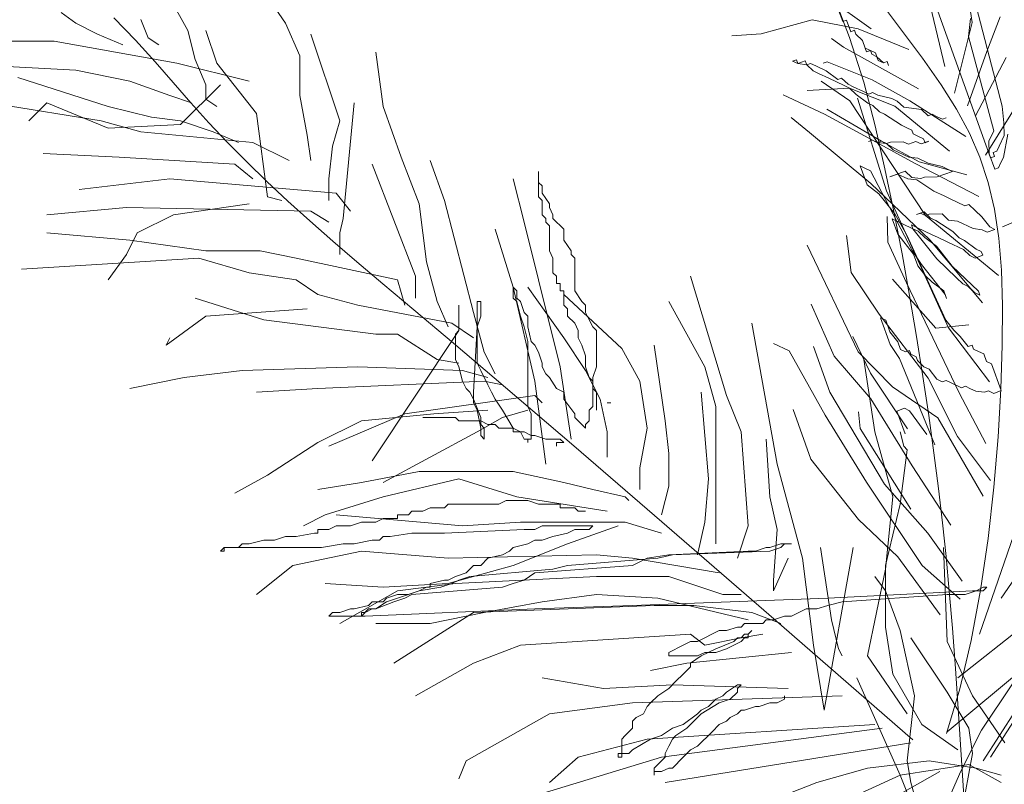
# Model space of a CAD drawing. Units: millimetres. Extents: x 595116 to 630915, y 909473 to 920225.
# Tile 22 of 134: x 629599.598 to 629606.562, y 919171.91 to 919177.315. Entities that reach past the tile are written whole.
import ezdxf

# ---------------------------------------------------------------- set-up
doc = ezdxf.new("R2010")
doc.units = ezdxf.units.MM
doc.layers.add('Dimension', color=3, linetype='Continuous', lineweight=18)
doc.layers.add('L-PLNT', color=85, linetype='Continuous', lineweight=13)
doc.styles.get("Standard").update_dxf_attribs({"font": 'arial.ttf'})
doc.dimstyles.new('ISO-25', dxfattribs={"dimtxt": 9, "dimasz": 6, "dimexe": 1.25, "dimexo": 0.625, "dimtad": 1, "dimlunit": 4, "dimtxsty": 'Standard', "dimcen": 2.5, "dimadec": 0, "dimazin": 0, "dimtfac": 1, "dimtmove": 0, "dimatfit": 3, "dimfxl": 1, "dimarcsym": 0})

# ---------------------------------------------------------------- blocks, each defined once
blk = doc.blocks.new('A$C4FB75ABC')
for p, q in [((2.7169, 3.7399), (2.6018, 4.2172)), ((2.8029, 3.5683), (2.5783, 4.1926)), ((1.2153, 3.9442), (1.2902, 3.808)), ((1.3924, 3.9442), (1.4742, 3.8217)), ((2.7679, 3.8231), (2.7507, 3.9385)), ((2.7636, 3.9026), (2.8247, 3.6653)), ((2.5777, 3.8114), (2.4796, 3.8815)), ((2.5372, 3.7949), (2.5035, 3.8821)), ((2.5794, 3.8826), (2.6314, 3.8136)), ((1.0518, 3.8421), (1.079, 3.8217)), ((2.5166, 3.8462), (2.5244, 3.8247)), ((1.1917, 3.7897), (1.1506, 3.8319)), ((1.2017, 3.8285), (1.2153, 3.7944)), ((2.4664, 3.8281), (2.3706, 3.8017)), ((2.5536, 3.8109), (2.4664, 3.8281)), ((2.5244, 3.8247), (2.5315, 3.8272)), ((2.5315, 3.8272), (2.5393, 3.8057)), ((2.7349, 3.6897), (2.7679, 3.8231)), ((2.7613, 3.7965), (2.7653, 3.8303)), ((2.7957, 3.7683), (2.8207, 3.834)), ((1.079, 3.8217), (1.1199, 3.8012)), ((1.2902, 3.808), (1.3039, 3.7536)), ((1.3243, 3.808), (1.3447, 3.7467)), ((1.4742, 3.8217), (1.5014, 3.7604)), ((2.5393, 3.8057), (2.5464, 3.8083)), ((2.5464, 3.8083), (2.549, 3.8011)), ((2.6486, 3.7721), (2.5536, 3.8109)), ((2.6314, 3.8136), (2.6743, 3.7558)), ((0.9428, 3.7876), (1.0382, 3.7876)), ((1.0382, 3.7876), (1.2698, 3.7467)), ((1.1199, 3.8012), (1.1676, 3.7808)), ((1.2284, 3.7492), (1.1917, 3.7897)), ((1.2153, 3.7944), (1.2357, 3.7808)), ((1.5219, 3.8012), (1.5764, 3.6378)), ((2.3706, 3.8017), (2.3152, 3.798)), ((2.5255, 3.7764), (2.5034, 3.7928)), ((2.5638, 3.7106), (2.5372, 3.7949)), ((2.549, 3.8011), (2.5614, 3.7893)), ((2.5614, 3.7893), (2.5665, 3.775)), ((2.8089, 3.6191), (2.7613, 3.7965)), ((1.6445, 3.7672), (1.6581, 3.665)), ((2.6672, 3.6978), (2.5255, 3.7764)), ((2.5665, 3.775), (2.5763, 3.7704)), ((2.5691, 3.7678), (2.5665, 3.775)), ((2.5763, 3.7704), (2.5691, 3.7678)), ((2.5763, 3.7704), (2.5789, 3.7632)), ((2.586, 3.7658), (2.5763, 3.7704)), ((2.7596, 3.6662), (2.7957, 3.7683)), ((1.2625, 3.7099), (1.2284, 3.7492)), ((1.3039, 3.7536), (1.3243, 3.7059)), ((1.5014, 3.7604), (1.5014, 3.6855)), ((2.4369, 3.7526), (2.4297, 3.7501)), ((2.4297, 3.7501), (2.4394, 3.7455)), ((2.4394, 3.7455), (2.4369, 3.7526)), ((2.4538, 3.7506), (2.4394, 3.7455)), ((2.4564, 3.7435), (2.4538, 3.7506)), ((2.4948, 3.7492), (2.4876, 3.7466)), ((2.58, 3.715), (2.4948, 3.7492)), ((2.5789, 3.7632), (2.5886, 3.7586)), ((2.5886, 3.7586), (2.586, 3.7658)), ((2.5886, 3.7586), (2.5912, 3.7515)), ((2.601, 3.7469), (2.5886, 3.7586)), ((2.5912, 3.7515), (2.601, 3.7469)), ((2.601, 3.7469), (2.6081, 3.7494)), ((2.6081, 3.7494), (2.601, 3.7469)), ((2.6081, 3.7494), (2.6107, 3.7423)), ((2.6107, 3.7423), (2.6081, 3.7494)), ((2.6743, 3.7558), (2.7096, 3.7056)), ((2.7745, 3.6472), (2.8322, 3.7571)), ((0.9496, 3.7399), (1.079, 3.7331)), ((1.079, 3.7331), (1.1812, 3.7127)), ((1.2698, 3.7467), (1.4061, 3.7127)), ((1.3447, 3.7467), (1.4197, 3.6514)), ((2.4394, 3.7455), (2.4564, 3.7435)), ((2.4635, 3.746), (2.4564, 3.7435)), ((2.4564, 3.7435), (2.4687, 3.7317)), ((2.4733, 3.7414), (2.4635, 3.746)), ((2.4687, 3.7317), (2.4785, 3.7271)), ((2.4928, 3.7323), (2.4733, 3.7414)), ((2.5149, 3.7159), (2.4928, 3.7323)), ((0.97, 3.7195), (1.1403, 3.665)), ((1.1812, 3.7127), (1.2562, 3.6855)), ((2.4785, 3.7271), (2.498, 3.7179)), ((2.5376, 3.6754), (2.4836, 3.7127)), ((2.498, 3.7179), (2.5272, 3.7041)), ((2.5221, 3.7185), (2.5149, 3.7159)), ((2.5344, 3.7067), (2.5221, 3.7185)), ((2.6509, 3.6757), (2.58, 3.715)), ((1.2959, 3.6716), (1.2625, 3.7099)), ((1.3515, 3.7059), (1.2766, 3.631)), ((1.3243, 3.7059), (1.3243, 3.6787)), ((2.537, 3.6995), (2.4575, 3.6952)), ((2.5272, 3.7041), (2.537, 3.6995)), ((2.5441, 3.7021), (2.5344, 3.7067)), ((2.537, 3.6995), (2.5493, 3.6877)), ((2.6222, 3.6653), (2.537, 3.6995)), ((2.5637, 3.6929), (2.5441, 3.7021)), ((2.5734, 3.6883), (2.5637, 3.6929)), ((2.5853, 3.6284), (2.5638, 3.7106)), ((2.7096, 3.7056), (2.7388, 3.6597)), ((1.2562, 3.6855), (1.297, 3.6718)), ((1.3243, 3.6787), (1.3447, 3.665)), ((1.5014, 3.6855), (1.5151, 3.6106)), ((2.4899, 3.6502), (2.4119, 3.6869)), ((2.6801, 3.4593), (2.5376, 3.6754)), ((2.5493, 3.6877), (2.5714, 3.6714)), ((2.6067, 3.5058), (2.5519, 3.6806)), ((2.5806, 3.6909), (2.5734, 3.6883)), ((2.5903, 3.6863), (2.5806, 3.6909)), ((2.617, 3.6797), (2.5903, 3.6863)), ((2.6268, 3.6751), (2.617, 3.6797)), ((2.6391, 3.6633), (2.6268, 3.6751)), ((2.7562, 3.6082), (2.6509, 3.6757)), ((2.7932, 3.5729), (2.8652, 3.6879)), ((0.9155, 3.6718), (1.1267, 3.6378)), ((1.0245, 3.6718), (0.9905, 3.6378)), ((1.1403, 3.6242), (1.0245, 3.6718)), ((1.1403, 3.665), (1.2221, 3.6446)), ((1.3299, 3.6341), (1.2959, 3.6716)), ((1.6036, 3.6718), (1.5832, 3.4539)), ((1.6581, 3.665), (1.6922, 3.5697)), ((2.5972, 3.5996), (2.4945, 3.6599)), ((2.5714, 3.6714), (2.5812, 3.6668)), ((2.5812, 3.6668), (2.5935, 3.655)), ((2.5935, 3.655), (2.6032, 3.6504)), ((2.7255, 3.5809), (2.6222, 3.6653)), ((2.673, 3.6593), (2.6391, 3.6633)), ((2.6853, 3.6475), (2.673, 3.6593)), ((2.7388, 3.6597), (2.763, 3.6147)), ((2.8247, 3.6653), (2.8279, 3.634)), ((1.1267, 3.6378), (1.2017, 3.6174)), ((1.2221, 3.6446), (1.2766, 3.6378)), ((1.2766, 3.6378), (1.3379, 3.6174)), ((1.4197, 3.6514), (1.4401, 3.4948)), ((1.5764, 3.6378), (1.5627, 3.5901)), ((2.4618, 3.6157), (2.4274, 3.6439)), ((2.5803, 3.6016), (2.4899, 3.6502)), ((2.6032, 3.6504), (2.6351, 3.6295)), ((2.6925, 3.6501), (2.6853, 3.6475)), ((2.7022, 3.6455), (2.6925, 3.6501)), ((2.712, 3.6409), (2.7022, 3.6455)), ((2.7192, 3.6435), (2.712, 3.6409)), ((1.2766, 3.631), (1.1403, 3.6242)), ((1.365, 3.5971), (1.3299, 3.6341)), ((2.6037, 3.5475), (2.5853, 3.6284)), ((2.6351, 3.6295), (2.6448, 3.6249)), ((2.6448, 3.6249), (2.6546, 3.6203)), ((2.6546, 3.6203), (2.6572, 3.6131)), ((2.7998, 3.5996), (2.8089, 3.6191)), ((2.8279, 3.634), (2.8285, 3.6099)), ((1.2017, 3.6174), (1.4129, 3.5969)), ((1.3379, 3.6174), (1.3856, 3.5969)), ((1.5151, 3.6106), (1.5219, 3.5629)), ((2.5774, 3.5196), (2.4618, 3.6157)), ((2.5803, 3.6016), (2.5731, 3.5991)), ((2.5731, 3.5991), (2.5803, 3.6016)), ((2.5901, 3.597), (2.5803, 3.6016)), ((2.5803, 3.6016), (2.5901, 3.597)), ((2.6609, 3.5577), (2.5803, 3.6016)), ((2.5972, 3.5996), (2.5901, 3.597)), ((2.607, 3.595), (2.5972, 3.5996)), ((2.6681, 3.5603), (2.5972, 3.5996)), ((2.6572, 3.6131), (2.6669, 3.6085)), ((2.6669, 3.6085), (2.6767, 3.6039)), ((2.6864, 3.5993), (2.6721, 3.5942)), ((2.6767, 3.6039), (2.6793, 3.5967)), ((2.6793, 3.5967), (2.6864, 3.5993)), ((2.763, 3.6147), (2.7827, 3.5691)), ((2.8003, 3.5755), (2.7998, 3.5996)), ((2.8285, 3.6099), (2.8193, 3.5904)), ((2.8356, 3.6125), (2.827, 3.5688)), ((1.4014, 3.5604), (1.365, 3.5971)), ((1.4129, 3.5969), (1.481, 3.5629)), ((1.5627, 3.5901), (1.5559, 3.5288)), ((2.5901, 3.597), (2.607, 3.595)), ((2.6142, 3.5976), (2.607, 3.595)), ((2.607, 3.595), (2.6193, 3.5833)), ((2.6383, 3.5982), (2.6142, 3.5976)), ((2.6193, 3.5833), (2.6486, 3.5695)), ((2.648, 3.5936), (2.6383, 3.5982)), ((2.6623, 3.5987), (2.648, 3.5936)), ((2.6721, 3.5942), (2.6623, 3.5987)), ((2.8193, 3.5904), (2.8147, 3.5806)), ((1.0177, 3.5765), (1.1608, 3.5697)), ((1.1608, 3.5697), (1.3788, 3.5561)), ((1.6922, 3.5697), (1.7263, 3.4812)), ((1.7467, 3.5629), (1.7739, 3.488)), ((2.6486, 3.5695), (2.6655, 3.5675)), ((2.6655, 3.5675), (2.685, 3.5583)), ((2.7827, 3.5691), (2.7983, 3.5216)), ((2.8107, 3.5468), (2.8003, 3.5755)), ((2.8101, 3.5709), (2.8029, 3.5683)), ((2.8147, 3.5806), (2.8075, 3.578)), ((2.8075, 3.578), (2.8101, 3.5709)), ((2.827, 3.5688), (2.8224, 3.5591)), ((1.3788, 3.5561), (1.4129, 3.5288)), ((1.4393, 3.5237), (1.4014, 3.5604)), ((1.6377, 3.5561), (1.7194, 3.345)), ((2.5671, 3.5483), (2.5573, 3.5529)), ((2.5573, 3.5529), (2.5703, 3.517)), ((2.5769, 3.5437), (2.5671, 3.5483)), ((2.6552, 3.3935), (2.5769, 3.5437)), ((2.6204, 3.467), (2.6037, 3.5475)), ((2.7805, 3.4954), (2.6609, 3.5577)), ((2.7579, 3.5359), (2.6681, 3.5603)), ((2.685, 3.5583), (2.7117, 3.5517)), ((2.7117, 3.5517), (2.7214, 3.5471)), ((2.7214, 3.5471), (2.7312, 3.5425)), ((2.8178, 3.5493), (2.8107, 3.5468)), ((2.8224, 3.5591), (2.8178, 3.5493)), ((1.0858, 3.5084), (1.2562, 3.5288)), ((1.2562, 3.5288), (1.5696, 3.5016)), ((1.5559, 3.5288), (1.5559, 3.488)), ((1.9034, 3.5288), (1.9238, 3.4471)), ((1.9511, 3.4948), (1.9511, 3.5425)), ((1.9511, 3.5425), (1.9511, 3.522)), ((2.642, 3.5428), (2.6133, 3.5325)), ((2.6133, 3.5325), (2.6276, 3.5376)), ((2.6276, 3.5376), (2.6471, 3.5284)), ((2.6543, 3.531), (2.642, 3.5428)), ((2.6471, 3.5284), (2.6641, 3.5264)), ((2.6712, 3.529), (2.6543, 3.531)), ((2.6641, 3.5264), (2.6959, 3.5055)), ((2.6784, 3.5316), (2.6712, 3.529)), ((2.7025, 3.5321), (2.6784, 3.5316)), ((2.7312, 3.5425), (2.7025, 3.5321)), ((1.4788, 3.4868), (1.4393, 3.5237)), ((1.9511, 3.522), (1.9579, 3.5152)), ((1.9579, 3.5152), (1.9579, 3.5016)), ((2.5703, 3.517), (2.5924, 3.5006)), ((2.6885, 3.4136), (2.5774, 3.5196)), ((2.7983, 3.5216), (2.81, 3.4712)), ((1.4401, 3.4948), (1.4674, 3.488)), ((1.5696, 3.5016), (1.5968, 3.4676)), ((1.7739, 3.488), (1.8285, 3.2769)), ((1.9579, 3.488), (1.9511, 3.4948)), ((1.9579, 3.5016), (1.9715, 3.4812)), ((1.9579, 3.4608), (1.9579, 3.488)), ((2.5924, 3.5006), (2.6222, 3.4627)), ((2.7237, 3.248), (2.6067, 3.5058)), ((2.6959, 3.5055), (2.7154, 3.4963)), ((2.7154, 3.4963), (2.7252, 3.4917)), ((2.7252, 3.4917), (2.7544, 3.4779)), ((2.8253, 3.4385), (2.9518, 3.4922)), ((1.0245, 3.4608), (1.1744, 3.4744)), ((1.1744, 3.4744), (1.5219, 3.4676)), ((1.4061, 3.4812), (1.263, 3.4608)), ((1.5201, 3.4494), (1.4788, 3.4868)), ((1.7263, 3.4812), (1.7399, 3.3722)), ((1.9715, 3.4812), (1.9715, 3.4744)), ((1.9715, 3.4744), (1.9783, 3.4608)), ((2.7544, 3.4779), (2.7616, 3.4805)), ((2.7616, 3.4805), (2.774, 3.4687)), ((2.81, 3.4712), (2.8183, 3.4166)), ((1.263, 3.4608), (1.1949, 3.4267)), ((1.5219, 3.4676), (1.5559, 3.4471)), ((1.5832, 3.4539), (1.5764, 3.4267)), ((1.9647, 3.4539), (1.9579, 3.4608)), ((1.9647, 3.4471), (1.9647, 3.4539)), ((1.9783, 3.4608), (1.9783, 3.4539)), ((1.9783, 3.4539), (1.9988, 3.4335)), ((2.609, 3.4093), (2.6078, 3.4576)), ((2.6566, 3.4346), (2.6176, 3.453)), ((2.6176, 3.453), (2.6279, 3.4243)), ((2.636, 3.3873), (2.6204, 3.467)), ((2.6222, 3.4627), (2.6449, 3.4222)), ((2.6632, 3.4613), (2.6776, 3.4664)), ((2.6704, 3.4639), (2.6632, 3.4613)), ((2.6801, 3.4593), (2.6704, 3.4639)), ((2.6776, 3.4664), (2.6899, 3.4547)), ((2.6873, 3.4618), (2.6801, 3.4593)), ((2.8178, 3.3467), (2.6801, 3.4593)), ((2.7114, 3.4624), (2.6873, 3.4618)), ((2.6899, 3.4547), (2.6996, 3.4501)), ((2.7237, 3.4506), (2.7114, 3.4624)), ((2.774, 3.4687), (2.7863, 3.4569)), ((2.7863, 3.4569), (2.8012, 3.438)), ((1.5633, 3.4112), (1.5201, 3.4494)), ((1.8693, 3.4335), (1.9034, 3.3246)), ((1.9238, 3.4471), (1.9511, 3.3382)), ((1.9715, 3.4403), (1.9647, 3.4471)), ((1.9715, 3.3927), (1.9715, 3.4403)), ((1.9988, 3.4335), (1.9988, 3.4131)), ((2.6638, 3.4372), (2.654, 3.4418)), ((2.654, 3.4418), (2.6566, 3.4346)), ((2.6566, 3.4346), (2.6664, 3.43)), ((2.6865, 3.3967), (2.6566, 3.4346)), ((2.693, 3.4234), (2.6638, 3.4372)), ((2.6996, 3.4501), (2.7315, 3.4291)), ((2.7407, 3.4486), (2.7237, 3.4506)), ((2.7699, 3.4348), (2.7407, 3.4486)), ((2.7869, 3.4328), (2.7699, 3.4348)), ((2.7966, 3.4282), (2.7869, 3.4328)), ((2.811, 3.4334), (2.7966, 3.4282)), ((2.8012, 3.438), (2.811, 3.4334)), ((1.0245, 3.4267), (1.1812, 3.4131)), ((1.1949, 3.4267), (1.1744, 3.3858)), ((1.5764, 3.4267), (1.5764, 3.3858)), ((2.5404, 3.3522), (2.5315, 3.422)), ((2.6279, 3.4243), (2.6578, 3.3864)), ((2.6449, 3.4222), (2.7186, 3.2624)), ((2.6664, 3.43), (2.6787, 3.4182)), ((2.6787, 3.4182), (2.7008, 3.4019)), ((2.7028, 3.4188), (2.693, 3.4234)), ((2.7223, 3.4096), (2.7028, 3.4188)), ((2.7315, 3.4291), (2.7438, 3.4173)), ((2.7438, 3.4173), (2.7536, 3.4127)), ((2.8183, 3.4166), (2.8233, 3.3565)), ((1.1812, 3.4131), (1.3243, 3.3927)), ((1.6088, 3.3721), (1.5633, 3.4112)), ((1.9988, 3.4131), (2.0124, 3.3927)), ((2.5536, 3.203), (2.4572, 3.4034)), ((2.6446, 3.333), (2.609, 3.4093)), ((2.7014, 3.3777), (2.6865, 3.3967)), ((2.7877, 3.2953), (2.6885, 3.4136)), ((2.7008, 3.4019), (2.7306, 3.364)), ((2.7516, 3.3958), (2.7223, 3.4096)), ((2.7639, 3.384), (2.7516, 3.3958)), ((2.7536, 3.4127), (2.7757, 3.3964)), ((2.7757, 3.3964), (2.7854, 3.3918)), ((0.9768, 3.3586), (1.3107, 3.379)), ((1.1744, 3.3858), (1.1403, 3.3382)), ((1.3107, 3.379), (1.4061, 3.3518)), ((1.3243, 3.3927), (1.4265, 3.3927)), ((1.4265, 3.3927), (1.4946, 3.379)), ((1.4946, 3.379), (1.6854, 3.3382)), ((1.9783, 3.379), (1.9715, 3.3927)), ((1.9783, 3.3518), (1.9783, 3.379)), ((2.0124, 3.3927), (2.0124, 3.3858)), ((2.0124, 3.3858), (2.0192, 3.379)), ((2.0192, 3.379), (2.0192, 3.3178)), ((2.6503, 3.3086), (2.636, 3.3873)), ((2.6727, 3.3674), (2.6552, 3.3935)), ((2.6578, 3.3864), (2.6655, 3.3648)), ((2.7384, 3.3424), (2.7014, 3.3777)), ((2.7737, 3.3794), (2.7639, 3.384)), ((2.788, 3.3846), (2.7737, 3.3794)), ((2.7854, 3.3918), (2.788, 3.3846)), ((1.6577, 3.3307), (1.6088, 3.3721)), ((1.7399, 3.3722), (1.7603, 3.2973)), ((2.6655, 3.3648), (2.6804, 3.3459)), ((2.7174, 3.3106), (2.6727, 3.3674)), ((2.7306, 3.364), (2.743, 3.3522)), ((1.4061, 3.3518), (1.4946, 3.3382)), ((1.7194, 3.345), (1.7194, 3.3041)), ((1.9851, 3.345), (1.9783, 3.3518)), ((1.9851, 3.3314), (1.9851, 3.345)), ((2.2372, 3.345), (2.3054, 3.1203)), ((2.5929, 3.2739), (2.5404, 3.3522)), ((2.6997, 3.2474), (2.6179, 3.3396)), ((2.6804, 3.3459), (2.6928, 3.3341)), ((2.7507, 3.3307), (2.7384, 3.3424)), ((2.743, 3.3522), (2.7553, 3.3404)), ((2.7553, 3.3404), (2.78, 3.3169)), ((2.8233, 3.3565), (2.8254, 3.2898)), ((1.4946, 3.3382), (1.5355, 3.3109)), ((1.7159, 3.2817), (1.6577, 3.3307)), ((1.6854, 3.3382), (1.699, 3.2905)), ((1.9102, 3.3178), (1.9034, 3.3246)), ((1.9034, 3.3246), (1.9034, 3.3041)), ((1.9034, 3.3246), (1.9443, 3.1475)), ((1.9306, 3.3246), (1.9988, 3.2292)), ((1.9511, 3.3382), (1.992, 3.1748)), ((1.992, 3.3314), (1.9851, 3.3314)), ((1.992, 3.3178), (1.992, 3.3314)), ((2.7435, 3.1255), (2.6446, 3.333)), ((2.6928, 3.3341), (2.7149, 3.3178)), ((2.7605, 3.3261), (2.7507, 3.3307)), ((2.7728, 3.3143), (2.7605, 3.3261)), ((1.3039, 3.3041), (1.4333, 3.2633)), ((1.5355, 3.3109), (1.6104, 3.2905)), ((1.9034, 3.3041), (1.9102, 3.2973)), ((1.9102, 3.3041), (1.9102, 3.3178)), ((1.917, 3.2973), (1.9102, 3.3041)), ((1.9988, 3.3178), (1.992, 3.3178)), ((1.9988, 3.2905), (1.9988, 3.3178)), ((1.9988, 3.3109), (2.1078, 3.2088)), ((2.0192, 3.3178), (2.0328, 3.2973)), ((2.6635, 3.2315), (2.6503, 3.3086)), ((2.7149, 3.3178), (2.72, 3.3034)), ((2.72, 3.3034), (2.7174, 3.3106)), ((2.7826, 3.3097), (2.7728, 3.3143)), ((2.78, 3.3169), (2.7826, 3.3097)), ((1.6104, 3.2905), (1.7876, 3.2565)), ((1.7603, 3.2973), (1.7808, 3.2497)), ((1.8012, 3.2429), (1.8012, 3.2905)), ((1.8012, 3.2905), (1.8012, 3.2429)), ((1.8421, 3.2973), (1.8353, 3.2973)), ((1.8353, 3.2973), (1.8353, 3.2497)), ((1.8421, 3.2701), (1.8421, 3.2973)), ((1.9102, 3.2973), (1.917, 3.2701)), ((1.9238, 3.2769), (1.917, 3.2973)), ((2.0056, 3.2837), (1.9988, 3.2905)), ((2.0328, 3.2973), (2.0396, 3.2905)), ((2.0396, 3.2905), (2.0396, 3.2769)), ((2.1963, 3.2973), (2.2645, 3.1748)), ((2.508, 3.1947), (2.4647, 3.2926)), ((2.8254, 3.2898), (2.825, 3.2153)), ((1.3243, 3.2701), (1.2494, 3.2156)), ((1.5151, 3.2837), (1.3243, 3.2701)), ((1.7906, 3.2188), (1.7159, 3.2817)), ((1.8285, 3.2769), (1.8489, 3.202)), ((1.8353, 3.2497), (1.8421, 3.2701)), ((1.917, 3.2701), (1.9238, 3.2497)), ((1.9306, 3.2701), (1.9238, 3.2769)), ((1.9306, 3.2497), (1.9306, 3.2701)), ((2.0056, 3.2701), (2.0056, 3.2837)), ((2.0192, 3.2565), (2.0056, 3.2701)), ((2.0396, 3.2769), (2.0465, 3.2633)), ((2.685, 3.153), (2.5929, 3.2739)), ((2.6053, 3.2621), (2.5955, 3.2667)), ((2.5955, 3.2667), (2.6136, 3.2165)), ((1.4333, 3.2633), (1.6445, 3.236)), ((1.7876, 3.2565), (1.8285, 3.2292)), ((1.8353, 3.2497), (1.8285, 3.1271)), ((1.8353, 3.1816), (1.8353, 3.2497)), ((1.9238, 3.2497), (1.9306, 3.2224)), ((1.9375, 3.2224), (1.9306, 3.2497)), ((2.026, 3.2429), (2.0192, 3.2565)), ((2.0465, 3.2633), (2.0533, 3.2497)), ((2.0533, 3.2497), (2.0601, 3.2429)), ((2.353, 3.2565), (2.4007, 2.9909)), ((2.613, 3.2406), (2.6053, 3.2621)), ((2.7622, 3.2537), (2.6997, 3.2474)), ((2.7186, 3.2624), (2.7335, 3.2434)), ((2.8009, 3.1461), (2.7237, 3.248)), ((1.2494, 3.2156), (1.2562, 3.2292)), ((1.8012, 3.2429), (1.6377, 2.9977)), ((1.6445, 3.236), (1.6854, 3.236)), ((1.6854, 3.236), (1.7603, 3.1884)), ((1.7944, 3.236), (1.8012, 3.2429)), ((1.7944, 3.1884), (1.7944, 3.236)), ((1.9988, 3.2292), (2.0396, 3.1679)), ((2.026, 3.2292), (2.026, 3.2429)), ((2.0328, 3.2156), (2.026, 3.2292)), ((2.0601, 3.2429), (2.0601, 3.1748)), ((2.5763, 3.1625), (2.5433, 3.2317)), ((2.6279, 3.2216), (2.613, 3.2406)), ((2.6754, 3.1561), (2.6635, 3.2315)), ((2.7335, 3.2434), (2.7458, 3.2316)), ((2.7458, 3.2316), (2.7608, 3.2127)), ((1.8887, 3.1355), (1.7906, 3.2188)), ((1.9306, 3.2224), (1.9306, 3.0999)), ((1.9443, 3.2156), (1.9375, 3.2224)), ((1.9511, 3.202), (1.9443, 3.2156)), ((2.0396, 3.1952), (2.0328, 3.2156)), ((2.1691, 3.2156), (2.1895, 3.0726)), ((2.4234, 3.2048), (2.3941, 3.2186)), ((2.5, 3.127), (2.469, 3.2131)), ((2.6136, 3.2165), (2.6311, 3.1904)), ((2.6331, 3.2073), (2.6279, 3.2216)), ((2.7608, 3.2127), (2.7679, 3.2153)), ((2.7679, 3.2153), (2.7705, 3.2081)), ((2.825, 3.2153), (2.8223, 3.1323)), ((1.8489, 3.202), (1.8693, 3.1611)), ((1.9579, 3.1816), (1.9511, 3.202)), ((2.0396, 3.1748), (2.0396, 3.1952)), ((2.1078, 3.2088), (2.1418, 3.1475)), ((2.4914, 3.0833), (2.4234, 3.2048)), ((2.5774, 3.1143), (2.508, 3.1947)), ((2.6179, 3.137), (2.5536, 3.203)), ((2.6428, 3.2027), (2.6331, 3.2073)), ((2.65, 3.2053), (2.6428, 3.2027)), ((2.6526, 3.1981), (2.65, 3.2053)), ((2.6624, 3.1935), (2.6526, 3.1981)), ((2.6649, 3.1863), (2.6624, 3.1935)), ((2.7705, 3.2081), (2.7803, 3.2035)), ((2.7803, 3.2035), (2.79, 3.1989)), ((2.79, 3.1989), (2.7952, 3.1846)), ((1.3924, 3.1679), (1.6104, 3.1748)), ((1.6104, 3.1748), (1.808, 3.1679)), ((1.7603, 3.1884), (1.8012, 3.1816)), ((1.8012, 3.1748), (1.7944, 3.1884)), ((1.808, 3.1475), (1.8012, 3.1748)), ((1.8421, 3.1679), (1.8353, 3.1816)), ((1.9579, 3.1748), (1.9579, 3.1816)), ((1.9647, 3.1611), (1.9579, 3.1748)), ((1.992, 3.1748), (2.0124, 3.0386)), ((2.0465, 3.1543), (2.0396, 3.1748)), ((2.0601, 3.1748), (2.0533, 3.1543)), ((2.2645, 3.1748), (2.2849, 3.0999)), ((2.5847, 3.0522), (2.5642, 3.1884)), ((2.6311, 3.1904), (2.6976, 3.0279)), ((2.6773, 3.1746), (2.6649, 3.1863)), ((2.687, 3.17), (2.6773, 3.1746)), ((2.7952, 3.1846), (2.8049, 3.18)), ((2.8049, 3.18), (2.823, 3.1297)), ((1.1812, 3.1339), (1.2834, 3.1543)), ((1.2834, 3.1543), (1.3924, 3.1679)), ((1.808, 3.1679), (1.8557, 3.1543)), ((1.8557, 3.1407), (1.8421, 3.1679)), ((1.9715, 3.1543), (1.9647, 3.1611)), ((1.9851, 3.1339), (1.9715, 3.1543)), ((2.0396, 3.1679), (2.0669, 3.1135)), ((2.0533, 3.1475), (2.0465, 3.1543)), ((2.0533, 3.1543), (2.0533, 3.0999)), ((2.6463, 3.058), (2.5763, 3.1625)), ((2.6863, 3.0831), (2.6754, 3.1561)), ((2.7019, 3.151), (2.687, 3.17)), ((1.5355, 3.1339), (1.8489, 3.1475)), ((1.8148, 3.1339), (1.808, 3.1475)), ((1.8489, 3.1475), (1.883, 3.1407)), ((1.8625, 3.1271), (1.8557, 3.1407)), ((2.0174, 3.0255), (1.8887, 3.1355)), ((1.9443, 3.1475), (1.9647, 2.9909)), ((2.0533, 3.1339), (2.0533, 3.1475)), ((2.1418, 3.1475), (2.1555, 3.059)), ((2.7037, 3.0787), (2.6179, 3.137)), ((2.7407, 3.0434), (2.685, 3.153)), ((2.7117, 3.1464), (2.7019, 3.151)), ((2.7189, 3.149), (2.7117, 3.1464)), ((2.7286, 3.1444), (2.7189, 3.149)), ((2.7481, 3.1352), (2.7286, 3.1444)), ((2.7553, 3.1378), (2.7481, 3.1352)), ((2.7651, 3.1332), (2.7553, 3.1378)), ((1.4197, 3.1271), (1.5355, 3.1339)), ((1.699, 3.0862), (1.9443, 3.1203)), ((1.8216, 3.1271), (1.8148, 3.1339)), ((1.8285, 3.1135), (1.8216, 3.1271)), ((1.8285, 3.1271), (1.8285, 3.1067)), ((1.8693, 3.1135), (1.8625, 3.1271)), ((1.9443, 3.1203), (1.9579, 3.1067)), ((1.9988, 3.1271), (1.9851, 3.1339)), ((1.9988, 3.1135), (1.9988, 3.1271)), ((2.0601, 3.1271), (2.0533, 3.1339)), ((2.0601, 3.093), (2.0601, 3.1271)), ((2.2577, 3.1271), (2.2713, 2.9637)), ((2.3054, 3.1203), (2.3326, 3.0522)), ((2.603, 2.9533), (2.5, 3.127)), ((2.794, 3.0302), (2.7435, 3.1255)), ((2.7748, 3.1286), (2.7651, 3.1332)), ((2.7917, 3.1266), (2.7748, 3.1286)), ((2.7823, 2.6709), (2.9389, 3.1271)), ((2.7989, 3.1292), (2.7917, 3.1266)), ((2.8087, 3.1246), (2.7989, 3.1292)), ((2.823, 3.1297), (2.8087, 3.1246)), ((2.8223, 3.1323), (2.817, 3.0425)), ((1.8421, 3.0794), (1.8285, 3.1135)), ((1.8285, 3.1067), (1.8353, 3.093)), ((1.883, 3.093), (1.8693, 3.1135)), ((1.9306, 3.0999), (1.9375, 3.0862)), ((2.0192, 3.0862), (1.9988, 3.1135)), ((2.0533, 3.0999), (2.0465, 3.093)), ((2.0669, 3.1135), (2.0805, 3.0522)), ((2.0873, 3.1067), (2.0805, 3.1067)), ((2.2849, 3.0999), (2.2849, 2.9024)), ((2.6552, 2.9883), (2.5774, 3.1143)), ((1.5559, 3.0249), (1.699, 3.0862)), ((1.7535, 3.0862), (1.6173, 3.0726)), ((1.8557, 3.093), (1.7535, 3.0862)), ((1.8353, 3.093), (1.8421, 3.059)), ((1.9034, 3.059), (1.883, 3.093)), ((1.883, 3.0794), (1.9306, 3.093)), ((1.9375, 3.0862), (1.9375, 3.0386)), ((2.0192, 3.0794), (2.0192, 3.0862)), ((2.0465, 3.093), (2.0465, 3.0726)), ((2.4644, 3.0007), (2.4308, 3.094)), ((2.5691, 2.9573), (2.4914, 3.0833)), ((2.5571, 3.0584), (2.5539, 3.0896)), ((2.6406, 3.0965), (2.6262, 3.0913)), ((2.6262, 3.0913), (2.6417, 3.0483)), ((2.6503, 3.0919), (2.6406, 3.0965)), ((2.6827, 3.0468), (2.6503, 3.0919)), ((2.696, 3.0126), (2.6863, 3.0831)), ((1.6173, 3.0726), (1.5355, 3.0318)), ((1.7331, 3.0794), (1.7944, 3.0794)), ((1.7944, 3.0794), (1.8012, 3.0726)), ((1.8012, 3.0726), (1.8421, 3.0726)), ((1.8353, 3.0522), (1.883, 3.0794)), ((1.8421, 3.0658), (1.8421, 3.0794)), ((1.8421, 3.0726), (1.8557, 3.0658)), ((1.8489, 3.059), (1.8421, 3.0658)), ((1.8557, 3.0658), (1.8693, 3.0658)), ((1.8693, 3.0658), (1.8761, 3.059)), ((2.0396, 3.059), (2.0192, 3.0794)), ((2.0465, 3.0726), (2.0396, 3.0658)), ((2.0396, 3.0658), (2.0396, 3.059)), ((2.1895, 3.0726), (2.1963, 3.0113)), ((2.7892, 2.9311), (2.7037, 3.0787)), ((1.6581, 2.9569), (1.8353, 3.0522)), ((1.8421, 3.059), (1.8421, 3.0454)), ((1.8421, 3.0454), (1.8489, 3.0386)), ((1.8489, 3.0386), (1.8489, 3.059)), ((1.8761, 3.059), (1.9034, 3.059)), ((1.917, 3.0522), (1.9034, 3.059)), ((1.9034, 3.059), (1.9034, 3.0522)), ((1.9034, 3.0522), (1.9238, 3.0522)), ((1.9238, 3.0386), (1.917, 3.0522)), ((1.9238, 3.0522), (1.9375, 3.0454)), ((1.9375, 3.0454), (1.9443, 3.0454)), ((1.9443, 3.0454), (1.9647, 3.0386)), ((2.0805, 3.0522), (2.0805, 3.0045)), ((2.1555, 3.059), (2.1418, 2.9841)), ((2.3326, 3.0522), (2.3462, 2.8751)), ((2.6523, 2.9062), (2.5571, 3.0584)), ((2.6187, 2.9296), (2.5847, 3.0522)), ((2.6392, 3.0249), (2.6324, 3.0522)), ((2.8029, 2.9604), (2.7407, 3.0434)), ((1.5355, 3.0318), (1.4401, 2.9705)), ((1.9306, 3.0386), (1.9238, 3.0386)), ((1.9375, 3.0386), (1.9306, 3.0386)), ((1.9306, 3.0386), (1.9306, 3.0318)), ((1.9306, 3.0318), (1.9306, 3.0386)), ((1.9647, 3.0386), (1.992, 3.0386)), ((1.9988, 3.0318), (1.9851, 3.0318)), ((1.9851, 3.0318), (1.9851, 3.0249)), ((1.992, 3.0386), (1.9988, 3.0318)), ((2.1835, 2.8826), (2.0174, 3.0255)), ((2.3803, 3.0386), (2.3871, 2.9296)), ((2.646, 3.0181), (2.6392, 3.0249)), ((2.817, 3.0425), (2.809, 2.948)), ((2.1963, 3.0113), (2.1963, 2.95)), ((2.6324, 2.916), (2.646, 3.0181)), ((2.7046, 2.9452), (2.696, 3.0126)), ((2.4007, 2.9909), (2.4484, 2.8139)), ((2.5539, 2.887), (2.4644, 3.0007)), ((2.7278, 2.8766), (2.6552, 2.9883)), ((1.4401, 2.9705), (1.3788, 2.9364)), ((1.6173, 2.9569), (1.7263, 2.9773)), ((1.7263, 2.9773), (1.9034, 2.9773)), ((1.9034, 2.9773), (1.9988, 2.9569)), ((2.1418, 2.9841), (2.1418, 2.9432)), ((1.5355, 2.9432), (1.6173, 2.9569)), ((1.8012, 2.9637), (1.6581, 2.9296)), ((1.9102, 2.9296), (1.8012, 2.9637)), ((1.9988, 2.9569), (2.0533, 2.9432)), ((2.1963, 2.95), (2.1827, 2.8956)), ((2.2713, 2.9637), (2.2645, 2.882)), ((2.6741, 2.8006), (2.5691, 2.9573)), ((2.6847, 2.8611), (2.603, 2.9533)), ((2.0533, 2.9432), (2.1146, 2.9296)), ((2.7122, 2.8807), (2.7046, 2.9452)), ((2.809, 2.948), (2.7981, 2.8512)), ((1.6581, 2.9296), (1.5491, 2.8956)), ((1.7808, 2.916), (1.7739, 2.9092)), ((1.8761, 2.916), (1.7808, 2.916)), ((1.8898, 2.9228), (1.8761, 2.916)), ((1.9306, 2.9228), (1.8898, 2.9228)), ((2.0805, 2.9024), (1.9102, 2.9296)), ((1.9511, 2.916), (1.9306, 2.9228)), ((1.992, 2.916), (1.9511, 2.916)), ((1.992, 2.9092), (1.992, 2.916)), ((2.1146, 2.9296), (2.1214, 2.9228)), ((2.3871, 2.9296), (2.4007, 2.8683)), ((2.6051, 2.7934), (2.6187, 2.9296)), ((2.6051, 2.8002), (2.6324, 2.916)), ((1.5491, 2.8956), (1.5082, 2.8751)), ((1.5696, 2.8956), (1.808, 2.8751)), ((1.6854, 2.8956), (1.6854, 2.8888)), ((1.7058, 2.8956), (1.6854, 2.8956)), ((1.7126, 2.9024), (1.7058, 2.8956)), ((1.7331, 2.9024), (1.7126, 2.9024)), ((1.7467, 2.9092), (1.7331, 2.9024)), ((1.7739, 2.9092), (1.7467, 2.9092)), ((2.0192, 2.9092), (1.992, 2.9092)), ((2.026, 2.9024), (2.0192, 2.9092)), ((2.0396, 2.9024), (2.026, 2.9024)), ((2.2849, 2.9024), (2.2849, 2.8411)), ((1.6173, 2.882), (1.5968, 2.8751)), ((1.6445, 2.882), (1.6173, 2.882)), ((1.6581, 2.8888), (1.6445, 2.882)), ((1.6854, 2.8888), (1.6581, 2.8888)), ((1.808, 2.8751), (1.917, 2.882)), ((1.917, 2.882), (2.1146, 2.882)), ((2.1146, 2.882), (2.1827, 2.8615)), ((2.3943, 2.7002), (2.1835, 2.8826)), ((2.2645, 2.882), (2.2508, 2.8207)), ((2.6279, 2.8164), (2.5539, 2.887)), ((2.7189, 2.8171), (2.7122, 2.8807)), ((2.8231, 2.739), (2.9253, 2.8888)), ((1.5287, 2.8615), (1.4946, 2.8547)), ((1.5355, 2.8615), (1.5287, 2.8615)), ((1.5559, 2.8683), (1.5355, 2.8683)), ((1.5355, 2.8683), (1.5355, 2.8615)), ((1.5696, 2.8751), (1.5559, 2.8683)), ((1.5968, 2.8751), (1.5696, 2.8751)), ((1.6718, 2.8547), (1.7126, 2.8615)), ((1.7126, 2.8615), (1.7739, 2.8615)), ((1.7739, 2.8615), (1.9238, 2.8683)), ((1.9238, 2.8683), (1.9443, 2.8683)), ((1.9443, 2.8683), (1.9579, 2.8751)), ((1.9579, 2.8751), (2.0533, 2.8751)), ((2.0056, 2.8615), (1.9783, 2.8547)), ((2.101, 2.8751), (2.0056, 2.8411)), ((2.0192, 2.8683), (2.0056, 2.8615)), ((2.0465, 2.8683), (2.0192, 2.8683)), ((2.0533, 2.8751), (2.0465, 2.8683)), ((2.3462, 2.8751), (2.3258, 2.8139)), ((2.4007, 2.8683), (2.3939, 2.773)), ((2.7496, 2.771), (2.6847, 2.8611)), ((1.3924, 2.8411), (1.3856, 2.8343)), ((1.4061, 2.8411), (1.3924, 2.8411)), ((1.4333, 2.8479), (1.4061, 2.8411)), ((1.4537, 2.8479), (1.4333, 2.8479)), ((1.4742, 2.8547), (1.4537, 2.8479)), ((1.4946, 2.8547), (1.4742, 2.8547)), ((1.5423, 2.8343), (1.5832, 2.8411)), ((1.5832, 2.8411), (1.6036, 2.8411)), ((1.6036, 2.8411), (1.6377, 2.8479)), ((1.6377, 2.8479), (1.6513, 2.8479)), ((1.6513, 2.8479), (1.6581, 2.8547)), ((1.6581, 2.8547), (1.6718, 2.8547)), ((1.9306, 2.8411), (1.9034, 2.8343)), ((2.0056, 2.8411), (1.9034, 2.8002)), ((1.9443, 2.8479), (1.9306, 2.8411)), ((1.9579, 2.8479), (1.9443, 2.8479)), ((1.9783, 2.8547), (1.9579, 2.8479)), ((2.3871, 2.8343), (2.4075, 2.8411)), ((2.4075, 2.8411), (2.428, 2.8411)), ((2.4144, 2.8411), (2.4075, 2.8343)), ((2.428, 2.8411), (2.4144, 2.8411)), ((2.7981, 2.8512), (2.784, 2.7542)), ((1.3515, 2.8275), (1.3584, 2.8343)), ((1.3584, 2.8275), (1.3515, 2.8275)), ((1.3856, 2.8343), (1.3584, 2.8343)), ((1.3584, 2.8343), (1.3584, 2.8275)), ((1.3584, 2.8343), (1.5423, 2.8343)), ((1.4878, 2.8002), (1.6173, 2.8275)), ((1.6173, 2.8275), (1.7808, 2.8139)), ((1.7808, 2.8139), (2.0601, 2.8207)), ((1.883, 2.8207), (1.8557, 2.8139)), ((1.8966, 2.8275), (1.883, 2.8207)), ((1.9034, 2.8343), (1.8966, 2.8275)), ((2.0601, 2.8207), (2.1282, 2.8139)), ((2.1555, 2.8139), (2.1963, 2.8207)), ((2.2032, 2.8207), (2.1759, 2.8139)), ((2.1963, 2.8207), (2.3462, 2.8275)), ((2.3871, 2.8275), (2.2032, 2.8207)), ((2.3462, 2.8275), (2.3599, 2.8275)), ((2.3599, 2.8275), (2.3803, 2.8343)), ((2.3803, 2.8343), (2.3871, 2.8343)), ((2.4075, 2.8343), (2.3871, 2.8275)), ((2.4825, 2.8343), (2.5029, 2.6981)), ((2.4893, 2.5279), (2.5438, 2.8343)), ((2.7209, 2.6572), (2.7141, 2.8343)), ((1.8557, 2.8139), (1.8421, 2.8002)), ((2.1759, 2.8139), (2.0056, 2.8002)), ((2.1282, 2.8002), (2.1555, 2.8139)), ((2.1282, 2.8139), (2.2917, 2.7866)), ((2.3939, 2.7526), (2.4212, 2.8139)), ((2.4484, 2.8139), (2.4689, 2.6504)), ((2.7077, 2.7073), (2.6279, 2.8164)), ((2.7251, 2.7519), (2.7189, 2.8171)), ((1.4197, 2.7458), (1.4878, 2.8002)), ((1.9034, 2.8002), (1.7808, 2.7662)), ((1.8148, 2.7866), (1.7944, 2.7798)), ((1.8285, 2.8002), (1.8148, 2.7866)), ((1.9783, 2.7934), (1.8216, 2.7798)), ((1.8421, 2.8002), (1.8285, 2.8002)), ((1.9238, 2.773), (1.9443, 2.7866)), ((1.9443, 2.7866), (2.1282, 2.8002)), ((2.0056, 2.8002), (1.9783, 2.7934)), ((2.5711, 2.63), (2.6051, 2.7934)), ((2.6051, 2.6845), (2.6051, 2.8002)), ((2.7456, 2.7371), (2.6741, 2.8006)), ((1.6581, 2.7594), (1.5491, 2.7662)), ((1.7808, 2.7662), (1.6581, 2.7594)), ((1.6854, 2.7526), (1.7944, 2.7662)), ((1.7739, 2.773), (1.7467, 2.7662)), ((1.7467, 2.7662), (1.7467, 2.7594)), ((1.7876, 2.7662), (1.7671, 2.7594)), ((1.7808, 2.773), (1.7739, 2.773)), ((1.7944, 2.7798), (1.7808, 2.773)), ((1.8012, 2.773), (1.7876, 2.7662)), ((1.7944, 2.7662), (2.0601, 2.7798)), ((1.8216, 2.7798), (1.8012, 2.773)), ((1.883, 2.7594), (1.9034, 2.7662)), ((1.9034, 2.7662), (1.9238, 2.773)), ((2.0601, 2.7798), (2.1078, 2.7798)), ((2.1078, 2.7798), (2.1963, 2.7798)), ((2.1963, 2.7798), (2.2985, 2.7458)), ((2.3939, 2.773), (2.3939, 2.7526)), ((2.6051, 2.7526), (2.5847, 2.7798)), ((1.5764, 2.6913), (1.6854, 2.7526)), ((1.7263, 2.7526), (1.6854, 2.739)), ((1.7263, 2.7526), (1.7058, 2.7458)), ((1.7126, 2.7458), (1.883, 2.7594)), ((1.7399, 2.7594), (1.7263, 2.7526)), ((1.7671, 2.7594), (1.7263, 2.7526)), ((1.7467, 2.7594), (1.7399, 2.7594)), ((2.4961, 2.739), (2.7686, 2.7526)), ((2.6324, 2.6777), (2.6051, 2.7526)), ((2.7309, 2.6826), (2.7251, 2.7519)), ((2.7754, 2.7526), (2.755, 2.7458)), ((2.784, 2.7542), (2.7664, 2.6591)), ((2.7686, 2.7526), (2.7891, 2.7526)), ((2.7891, 2.7594), (2.7754, 2.7526)), ((2.7891, 2.7526), (2.7959, 2.7594)), ((2.7959, 2.7594), (2.7891, 2.7594)), ((1.6377, 2.7321), (1.6309, 2.7253)), ((1.6581, 2.7321), (1.6377, 2.7321)), ((1.6649, 2.7321), (1.6445, 2.7185)), ((1.6445, 2.7185), (1.6786, 2.7321)), ((1.6649, 2.739), (1.6581, 2.7321)), ((1.6854, 2.7458), (1.6649, 2.739)), ((1.6854, 2.739), (1.6649, 2.7321)), ((1.6786, 2.7321), (1.699, 2.739)), ((1.7058, 2.7458), (1.6854, 2.7458)), ((1.699, 2.739), (1.7126, 2.7458)), ((1.9579, 2.7321), (1.8489, 2.7117)), ((2.0601, 2.7458), (1.9579, 2.7321)), ((2.1759, 2.739), (2.0601, 2.7458)), ((2.1282, 2.7253), (2.3122, 2.7321)), ((2.3462, 2.6981), (2.1759, 2.739)), ((2.2985, 2.7458), (2.3326, 2.7458)), ((2.3122, 2.7321), (2.4961, 2.739)), ((2.5234, 2.7321), (2.4961, 2.7253)), ((2.7209, 2.7458), (2.5234, 2.7321)), ((2.755, 2.7458), (2.7209, 2.7458)), ((1.5627, 2.7117), (1.5559, 2.7049)), ((1.5764, 2.7117), (1.5627, 2.7117)), ((1.5968, 2.7185), (1.5764, 2.7117)), ((1.6036, 2.7185), (1.5968, 2.7185)), ((1.6309, 2.7253), (1.6036, 2.7185)), ((1.6309, 2.7185), (1.6173, 2.7049)), ((1.6173, 2.7049), (1.6173, 2.7117)), ((1.6173, 2.7117), (1.6241, 2.7117)), ((1.6241, 2.7117), (1.6377, 2.7185)), ((1.6241, 2.7049), (1.9443, 2.7185)), ((1.6445, 2.7185), (1.6309, 2.7185)), ((1.6377, 2.7185), (1.6445, 2.7185)), ((1.6786, 2.6164), (1.8285, 2.7117)), ((1.8489, 2.7117), (1.7467, 2.6913)), ((1.8285, 2.7117), (2.1691, 2.7253)), ((1.9443, 2.7185), (2.1282, 2.7253)), ((2.1691, 2.7253), (2.244, 2.7253)), ((2.244, 2.7253), (2.353, 2.7117)), ((2.353, 2.7117), (2.4075, 2.6913)), ((2.4552, 2.7185), (2.428, 2.7049)), ((2.4757, 2.7185), (2.4552, 2.7185)), ((2.4961, 2.7253), (2.4757, 2.7185)), ((2.7414, 2.5891), (2.9049, 2.7185)), ((1.5559, 2.7049), (1.6241, 2.7049)), ((1.7467, 2.6913), (1.6445, 2.6913)), ((2.3394, 2.6913), (2.3326, 2.6845)), ((2.3735, 2.6913), (2.3394, 2.6913)), ((2.3803, 2.6981), (2.3735, 2.6913)), ((2.3939, 2.6981), (2.3803, 2.6981)), ((2.4144, 2.7049), (2.3939, 2.6981)), ((2.6566, 2.472), (2.3943, 2.7002)), ((2.428, 2.7049), (2.4144, 2.7049)), ((2.5029, 2.6981), (2.5166, 2.6436)), ((2.2917, 2.6777), (2.2508, 2.6572)), ((2.3054, 2.6777), (2.2917, 2.6777)), ((2.3258, 2.6845), (2.3054, 2.6777)), ((2.3326, 2.6845), (2.3258, 2.6845)), ((2.3462, 2.6709), (2.353, 2.6777)), ((2.353, 2.6777), (2.3462, 2.6709)), ((2.6187, 2.596), (2.6051, 2.6845)), ((2.6596, 2.5551), (2.6324, 2.6777)), ((2.7367, 2.6065), (2.7309, 2.6826)), ((1.917, 2.6504), (2.2372, 2.6709)), ((2.2372, 2.6572), (2.2236, 2.6504)), ((2.2372, 2.6709), (2.2645, 2.6504)), ((2.2508, 2.6572), (2.2372, 2.6572)), ((2.2645, 2.6504), (2.3326, 2.664)), ((2.319, 2.6572), (2.2849, 2.6436)), ((2.3054, 2.6436), (2.3326, 2.6572)), ((2.3258, 2.664), (2.319, 2.6572)), ((2.3326, 2.664), (2.3258, 2.664)), ((2.3394, 2.6709), (2.3326, 2.664)), ((2.3326, 2.664), (2.3735, 2.6709)), ((2.3326, 2.6572), (2.3394, 2.664)), ((2.3462, 2.6709), (2.3394, 2.6709)), ((2.3394, 2.664), (2.3462, 2.664)), ((2.3462, 2.664), (2.3462, 2.6709)), ((2.6528, 2.664), (2.7209, 2.5619)), ((2.7209, 2.487), (2.9253, 2.6572)), ((2.7686, 2.5551), (2.7209, 2.6572)), ((2.7664, 2.6591), (2.7451, 2.5683)), ((1.8285, 2.6164), (1.917, 2.6504)), ((2.2236, 2.6504), (2.1963, 2.6368)), ((2.1963, 2.6368), (2.1963, 2.63)), ((2.428, 2.6368), (2.2304, 2.6164)), ((2.2508, 2.63), (2.2645, 2.6368)), ((2.2849, 2.6436), (2.2577, 2.63)), ((2.2645, 2.6368), (2.2849, 2.6368)), ((2.2849, 2.6368), (2.3054, 2.6436)), ((2.4689, 2.6504), (2.4893, 2.5279)), ((2.5166, 2.6436), (2.5234, 2.63)), ((1.7194, 2.5551), (1.8285, 2.6164)), ((2.2304, 2.6164), (2.1623, 2.6028)), ((2.1963, 2.63), (2.2508, 2.63)), ((2.2577, 2.63), (2.2372, 2.6164)), ((2.2372, 2.6164), (2.2372, 2.6096)), ((2.646, 2.5211), (2.5711, 2.63)), ((2.2372, 2.6096), (2.2236, 2.596)), ((2.7426, 2.5213), (2.7367, 2.6065)), ((2.0737, 2.5687), (1.9579, 2.5891)), ((2.21, 2.5823), (2.1963, 2.5687)), ((2.2236, 2.596), (2.21, 2.5823)), ((2.5506, 2.5891), (2.6324, 2.4053)), ((2.6732, 2.5006), (2.6187, 2.596)), ((2.2032, 2.5755), (2.0737, 2.5687)), ((2.1963, 2.5687), (2.1759, 2.5551)), ((2.4212, 2.5687), (2.2032, 2.5755)), ((2.2985, 2.5551), (2.3054, 2.5619)), ((2.3054, 2.5619), (2.3258, 2.5755)), ((2.3258, 2.5619), (2.3122, 2.5483)), ((2.3258, 2.5755), (2.3326, 2.5755)), ((2.3326, 2.5755), (2.3258, 2.5687)), ((2.3258, 2.5687), (2.3258, 2.5619)), ((2.7451, 2.5683), (2.72, 2.484)), ((2.7209, 2.5619), (2.7618, 2.4938)), ((2.786, 2.4905), (2.8442, 2.5778)), ((2.5234, 2.5551), (2.1282, 2.5415)), ((2.1759, 2.5551), (2.1623, 2.5415)), ((2.2781, 2.5415), (2.2849, 2.5483)), ((2.2849, 2.5483), (2.2985, 2.5551)), ((2.3122, 2.5483), (2.2917, 2.5415)), ((2.4007, 2.5415), (2.4144, 2.5483)), ((2.4144, 2.5483), (2.4144, 2.5551)), ((2.646, 2.4325), (2.6596, 2.5551)), ((2.8299, 2.4666), (2.7686, 2.5551)), ((2.1282, 2.5415), (1.9715, 2.5211)), ((2.1555, 2.5347), (2.1487, 2.5211)), ((2.1623, 2.5415), (2.1555, 2.5347)), ((2.2508, 2.5211), (2.2577, 2.5279)), ((2.2917, 2.5415), (2.2577, 2.5211)), ((2.2577, 2.5279), (2.2713, 2.5347)), ((2.2713, 2.5347), (2.2781, 2.5415)), ((2.3258, 2.5211), (2.3326, 2.5279)), ((2.3326, 2.5279), (2.3394, 2.5279)), ((2.3394, 2.5279), (2.3599, 2.5347)), ((2.3599, 2.5347), (2.3667, 2.5347)), ((2.3667, 2.5347), (2.3871, 2.5415)), ((2.3871, 2.5415), (2.4007, 2.5415)), ((2.7891, 2.4325), (2.8504, 2.5279)), ((2.8027, 2.4393), (2.864, 2.5347)), ((1.9715, 2.5211), (1.8148, 2.4325)), ((2.135, 2.5142), (2.1282, 2.5074)), ((2.1282, 2.5074), (2.1282, 2.4938)), ((2.1487, 2.5211), (2.135, 2.5142)), ((2.2236, 2.5006), (2.2508, 2.5211)), ((2.244, 2.5074), (2.2304, 2.4938)), ((2.2577, 2.5211), (2.244, 2.5074)), ((2.2917, 2.5006), (2.3054, 2.5074)), ((2.3054, 2.5074), (2.3122, 2.5142)), ((2.3122, 2.5142), (2.3258, 2.5211)), ((2.7489, 2.4244), (2.7426, 2.5213)), ((2.1282, 2.4938), (2.1146, 2.4802)), ((2.5847, 2.5006), (2.1555, 2.4734)), ((2.1827, 2.4802), (2.2032, 2.4938)), ((2.5983, 2.4938), (2.1827, 2.4393)), ((2.2032, 2.4938), (2.2236, 2.5006)), ((2.2304, 2.4938), (2.21, 2.4802)), ((2.2508, 2.4598), (2.2781, 2.487)), ((2.2781, 2.487), (2.2917, 2.5006)), ((2.7414, 2.453), (2.6732, 2.5006)), ((2.7471, 2.4129), (2.786, 2.4905)), ((2.7618, 2.4938), (2.7686, 2.4461)), ((2.1555, 2.4734), (2.026, 2.4393)), ((2.1146, 2.4802), (2.1078, 2.4734)), ((2.1078, 2.4734), (2.1078, 2.4461)), ((2.1282, 2.453), (2.1623, 2.4734)), ((2.1623, 2.4734), (2.1827, 2.4802)), ((2.2032, 2.4734), (2.1963, 2.4598)), ((2.21, 2.4802), (2.2032, 2.4734)), ((2.1214, 2.4461), (2.1282, 2.453)), ((2.6528, 2.4666), (2.1895, 2.3917)), ((2.1963, 2.4598), (2.1895, 2.4461)), ((2.2236, 2.4393), (2.2372, 2.453)), ((2.2372, 2.453), (2.2508, 2.4598)), ((1.8148, 2.4325), (1.8012, 2.3985)), ((2.1827, 2.4393), (1.9579, 2.3712)), ((2.026, 2.4393), (1.9715, 2.3917)), ((2.1078, 2.4461), (2.101, 2.4461)), ((2.101, 2.4461), (2.101, 2.4393)), ((2.101, 2.4393), (2.1078, 2.4393)), ((2.1078, 2.4393), (2.1078, 2.4461)), ((2.1078, 2.4461), (2.1214, 2.4461)), ((2.1895, 2.4393), (2.1759, 2.4257)), ((2.1895, 2.4461), (2.1895, 2.4393)), ((2.2032, 2.4189), (2.2236, 2.4393)), ((2.5711, 2.4189), (2.6869, 2.4325)), ((2.6528, 2.3917), (2.646, 2.4325)), ((2.6869, 2.4325), (2.7754, 2.4189)), ((2.7686, 2.4461), (2.755, 2.3712)), ((2.1759, 2.4257), (2.1691, 2.4189)), ((2.1691, 2.4189), (2.1691, 2.4053)), ((2.1691, 2.4053), (2.1691, 2.4121)), ((2.1691, 2.4121), (2.1827, 2.4121)), ((2.1827, 2.4121), (2.1963, 2.4189)), ((2.1963, 2.4189), (2.2032, 2.4189)), ((2.4757, 2.3917), (2.5711, 2.4189)), ((2.7073, 2.4121), (2.5983, 2.3508)), ((2.6324, 2.4053), (2.7618, 2.4257)), ((2.7083, 2.3255), (2.7471, 2.4129)), ((2.7559, 2.3132), (2.7489, 2.4244)), ((2.7618, 2.4257), (2.8231, 2.3917)), ((2.7754, 2.4189), (2.8231, 2.4053)), ((2.4825, 2.3372), (2.6324, 2.4053)), ((2.6324, 2.4053), (2.7073, 2.2214)), ((2.353, 2.344), (2.4757, 2.3917)), ((2.6732, 2.3168), (2.6528, 2.3917))]:
    blk.add_line(p, q)
blk = doc.blocks.new('*D216')
at = {"layer": 'Defpoints', "color": 0, "transparency": 16777216}
for p in [(629743.5408, 919411.9276), (629505.0408, 919411.8279), (629743.5408, 918832.3776)]:
    blk.add_point(p, dxfattribs=at)
at = {"layer": 'Dimension', "color": 0, "lineweight": -2, "transparency": 16777216}
for p, q in [((629743.5408, 919411.3026), (629743.5408, 918831.1276)), ((629505.0408, 919411.2029), (629505.0408, 918831.1276)), ((629511.0408, 918832.3776), (629737.5408, 918832.3776))]:
    blk.add_line(p, q, dxfattribs=at)
at = {"layer": 'Dimension', "color": 0, "transparency": 16777216}
for points in [[(629511.0408, 918833.3776), (629511.0408, 918831.3776), (629505.0408, 918832.3776)], [(629737.5408, 918833.3776), (629737.5408, 918831.3776), (629743.5408, 918832.3776)]]:
    blk.add_solid(points, dxfattribs=at)
at = {"layer": 'Dimension', "color": 0, "transparency": 16777216, "insert": (629624.2908, 918837.656), "char_height": 9, "attachment_point": 5}
blk.add_mtext('19\'-10 1/2"', dxfattribs=at)

msp = doc.modelspace()

# ---------------------------------------------------------------- block references
at = {"layer": 'L-PLNT', "xscale": 3.753413438031968, "yscale": 3.753413438031968, "zscale": 3.753413438031968}
msp.add_blockref('A$C4FB75ABC', (629595.9442, 919162.9458), dxfattribs=at)

# ---------------------------------------------------------------- dimensions: what is measured, and where the dimension line sits
at = {"layer": 'Dimension'}
dim = msp.add_linear_dim(base=(629743.5408, 918832.3776), p1=(629505.0408, 919411.8279), p2=(629743.5408, 919411.9276), dimstyle='ISO-25', override={"dimdec": 1, "dimlfac": 1, "dimrnd": 0, "dimzin": 1, "dimdsep": 46, "dimlunit": 4, "dimfrac": 2}, dxfattribs=at)
dim.commit()
dim.dimension.update_dxf_attribs({"geometry": '*D216', "text_midpoint": (629624.2908, 918837.656)})

doc.saveas('drawing.dxf')
